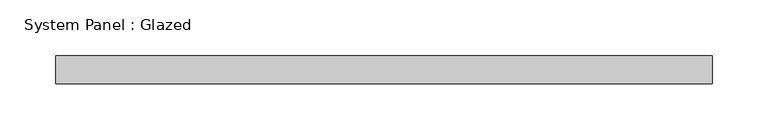
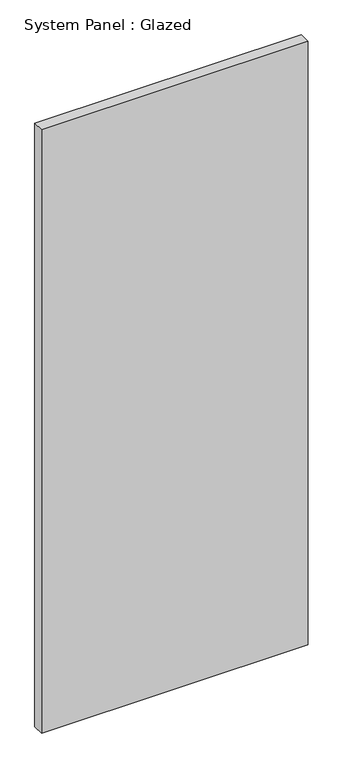
"""IFC4 building model written with IfcOpenShell, lengths in millimetres: plate geometry, System Panel : Glazed."""

from ifc_helpers import new_model, si_unit, origin, origin_with_axes, place, context, project, spatial, polyline, outline, extrude, source, transform, mapped, element, save


def system_panel_glazed_7e062a48(model_context):
    return source(origin(), model_context, "Body", "SweptSolid", [
        extrude(outline(polyline([(295.275, 19.05), (-295.275, 19.05), (-295.275, 44.45), (295.275, 44.45), (295.275, 19.05)])), origin_with_axes(), (0.0, 0.0, 1.0), 1412.437083),
    ])


if __name__ == "__main__":
    model = new_model("IFC4")
    model_context = context("Model", 3, world=origin())
    ifc_project = project(units=[si_unit("LENGTHUNIT", "METRE", prefix="MILLI")], contexts=[model_context])
    site = spatial("IfcSite", under=ifc_project)
    building = spatial("IfcBuilding", under=site)
    placement = place(None, origin())
    system_panel_glazed_shape = system_panel_glazed_7e062a48(model_context)
    element("IfcPlate", 1, ObjectType="System Panel : Glazed", at=placement, inside=building, context=model_context, shape_type="MappedRepresentation", body=[
        mapped(system_panel_glazed_shape, transform((0.0, 0.0, 0.0), x_axis=(1.0, 0.0, 0.0), y_axis=(0.0, 1.0, 0.0), z_axis=(0.0, 0.0, 1.0))),
    ])
    save(model, "model.ifc")

# Revit data of these elements
# Type "System Panel : Glazed"
#   Construction Type Id = "GSP4R"
#   Analytic Construction = "1/8 in Pilkington single glazing"
#   Visual Light Transmittance = 0.9
#   Solar Heat Gain Coefficient = 0.86
#   Heat Transfer Coefficient (U) = 1.18115 BTU/(h·ft²·°F)
#   Define Thermal Properties by = 1
# Element 1 (IfcPlate, "System Panel : Glazed")
#   Materials on its faces: "Glass"
# Materials
#   "Glass": class "Glass", colour RGB 0 128 192, transparency 0.75, Description = "Soda Lime Glass", Cost = 0
